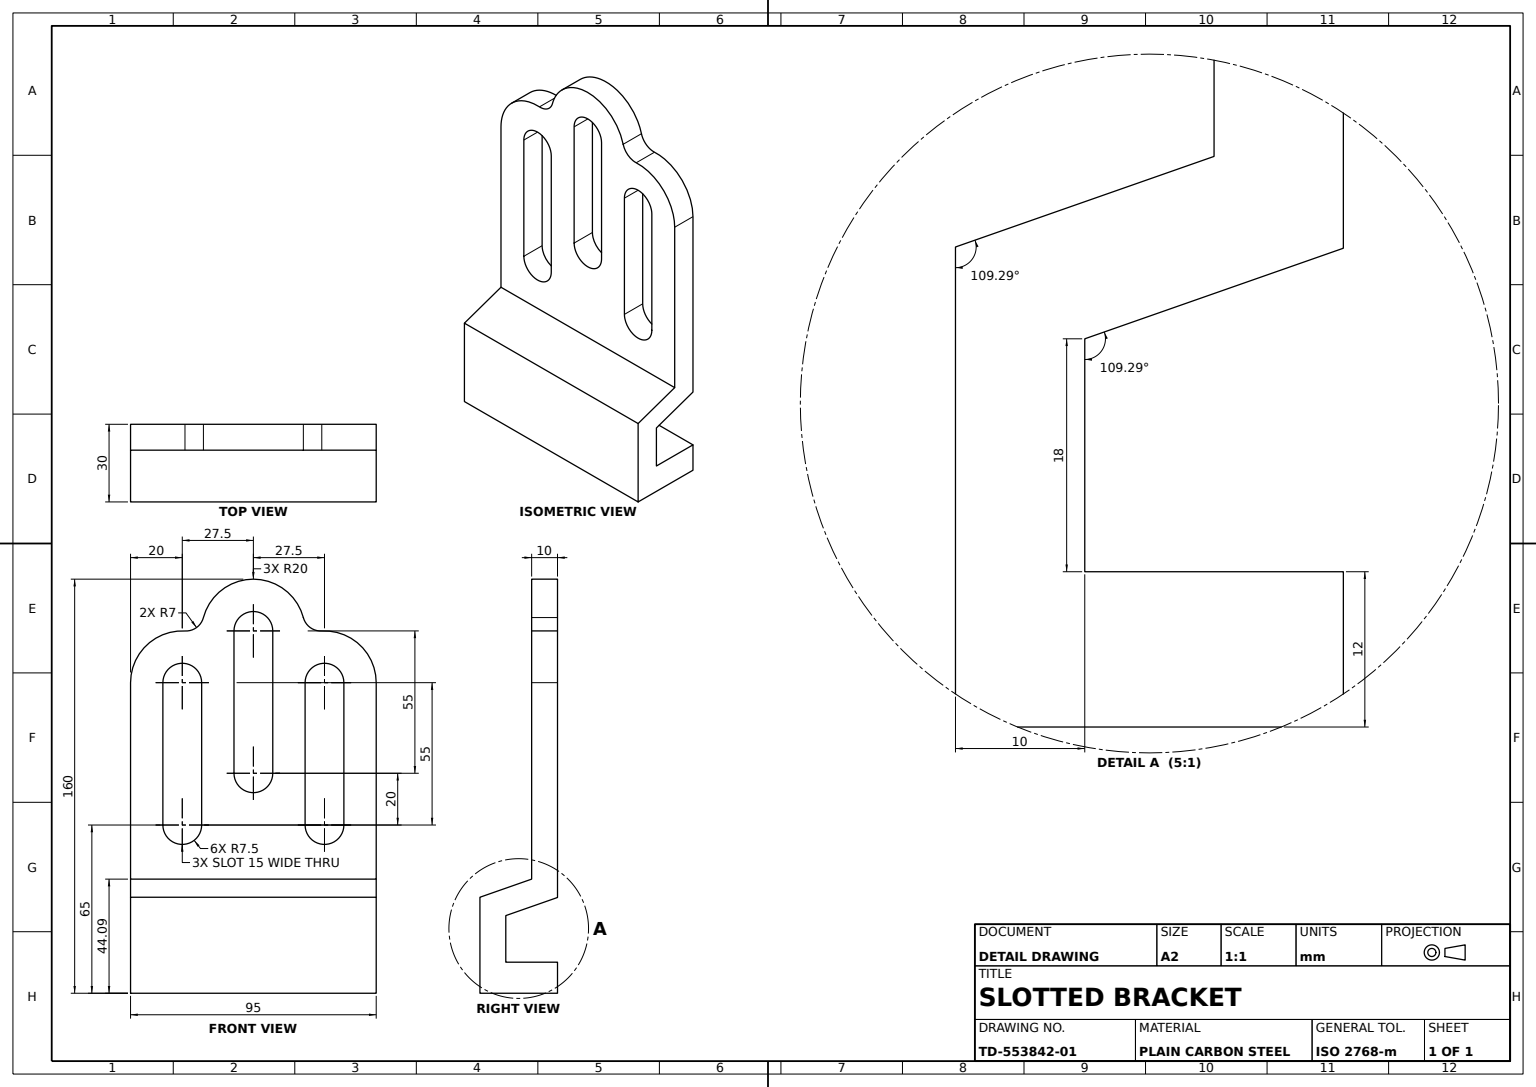
from build123d import *

# Parameters (mm, degrees)
SUPPORT_BODY_DEPTH         = 47.5
MOUNTING_SLOTS_3X7MM_REACH = 170.096


with BuildPart() as part:
    # Support Profile Sketch → Support Body (new, symmetric)
    with BuildSketch(Plane.XY):
        Polygon((-30, 0), (0, 0), (0, 37.09481005), (-20, 44.09481005), (-20, 160), (-30, 160), (-30, 37), (-10, 30), (-10, 12), (-30, 12), align=None)
    extrude(amount=SUPPORT_BODY_DEPTH, both=True)

    # Mounting Slots Sketch → Mounting Slots 3x7mm (cut, up to next)
    with BuildSketch(Plane(origin=(-20, 0, 0), x_dir=(0, 0, -1), z_dir=(1, 0, 0)), mode=Mode.PRIVATE) as mounting_slots_3x7mm_sk1:
        with BuildLine():
            Line((-35, 120), (-35, 65))
            ThreePointArc((-35, 65), (-27.5, 57.5), (-20, 65))
            Line((-20, 65), (-20, 120))
            ThreePointArc((-20, 120), (-27.5, 127.5), (-35, 120))
        make_face()
    mounting_slots_3x7mm_tool1 = extrude(mounting_slots_3x7mm_sk1.sketch, amount=-MOUNTING_SLOTS_3X7MM_REACH, mode=Mode.PRIVATE) & part.part
    # Mounting Slots Sketch → Mounting Slots 3x7mm (cut, up to next)
    with BuildSketch(Plane(origin=(-20, 0, 0), x_dir=(0, 0, -1), z_dir=(1, 0, 0)), mode=Mode.PRIVATE) as mounting_slots_3x7mm_sk2:
        with BuildLine():
            Line((-7.5, 140), (-7.5, 85))
            ThreePointArc((-7.5, 85), (0, 77.5), (7.5, 85))
            Line((7.5, 85), (7.5, 140))
            ThreePointArc((7.5, 140), (0, 147.5), (-7.5, 140))
        make_face()
    mounting_slots_3x7mm_tool2 = extrude(mounting_slots_3x7mm_sk2.sketch, amount=-MOUNTING_SLOTS_3X7MM_REACH, mode=Mode.PRIVATE) & part.part
    # Mounting Slots Sketch → Mounting Slots 3x7mm (cut, up to next)
    with BuildSketch(Plane(origin=(-20, 0, 0), x_dir=(0, 0, -1), z_dir=(1, 0, 0)), mode=Mode.PRIVATE) as mounting_slots_3x7mm_sk3:
        with BuildLine():
            ThreePointArc((35, 65), (27.5, 57.5), (20, 65))
            Line((20, 65), (20, 120))
            ThreePointArc((20, 120), (27.5, 127.5), (35, 120))
            Line((35, 120), (35, 65))
        make_face()
    mounting_slots_3x7mm_tool3 = extrude(mounting_slots_3x7mm_sk3.sketch, amount=-MOUNTING_SLOTS_3X7MM_REACH, mode=Mode.PRIVATE) & part.part
    # Mounting Slots Sketch → Mounting Slots 3x7mm (cut, up to next)
    with BuildSketch(Plane(origin=(-20, 0, 0), x_dir=(0, 0, -1), z_dir=(1, 0, 0)), mode=Mode.PRIVATE) as mounting_slots_3x7mm_sk4:
        with BuildLine():
            ThreePointArc((26.453123952, 139.97258247), (41.267034521, 134.507541504), (47.5, 120))
            Line((47.5, 120), (47.5, 160))
            Line((47.5, 160), (1.13e-07, 160))
            ThreePointArc((1.13e-07, 160), (12.182870127, 155.861200316), (19.323494322, 145.157767656))
            ThreePointArc((19.323494322, 145.157767656), (21.969515451, 141.301833745), (26.453123952, 139.97258247))
        make_face()
    mounting_slots_3x7mm_tool4 = extrude(mounting_slots_3x7mm_sk4.sketch, amount=-MOUNTING_SLOTS_3X7MM_REACH, mode=Mode.PRIVATE) & part.part
    # Mounting Slots Sketch → Mounting Slots 3x7mm (cut, up to next)
    with BuildSketch(Plane(origin=(-20, 0, 0), x_dir=(0, 0, -1), z_dir=(1, 0, 0)), mode=Mode.PRIVATE) as mounting_slots_3x7mm_sk5:
        with BuildLine():
            ThreePointArc((-19.323494322, 145.157767656), (-12.182870037, 155.861200385), (1.13e-07, 160))
            Line((1.13e-07, 160), (-47.5, 160))
            Line((-47.5, 160), (-47.5, 120))
            ThreePointArc((-47.5, 120), (-41.267034521, 134.507541504), (-26.453123952, 139.97258247))
            ThreePointArc((-26.453123952, 139.97258247), (-21.969515451, 141.301833745), (-19.323494322, 145.157767656))
        make_face()
    mounting_slots_3x7mm_tool5 = extrude(mounting_slots_3x7mm_sk5.sketch, amount=-MOUNTING_SLOTS_3X7MM_REACH, mode=Mode.PRIVATE) & part.part
    add(mounting_slots_3x7mm_tool1.solids().sort_by_distance((-20, 92.5, 27.5))[0], mode=Mode.SUBTRACT)
    add(mounting_slots_3x7mm_tool2.solids().sort_by_distance((-20, 112.5, 0))[0], mode=Mode.SUBTRACT)
    add(mounting_slots_3x7mm_tool3.solids().sort_by_distance((-20, 92.5, -27.5))[0], mode=Mode.SUBTRACT)
    add(mounting_slots_3x7mm_tool4.solids().sort_by_distance((-20, 149.008344, -32.791963))[0], mode=Mode.SUBTRACT)
    add(mounting_slots_3x7mm_tool5.solids().sort_by_distance((-20, 149.008344, 32.791963))[0], mode=Mode.SUBTRACT)


solid = part.part
